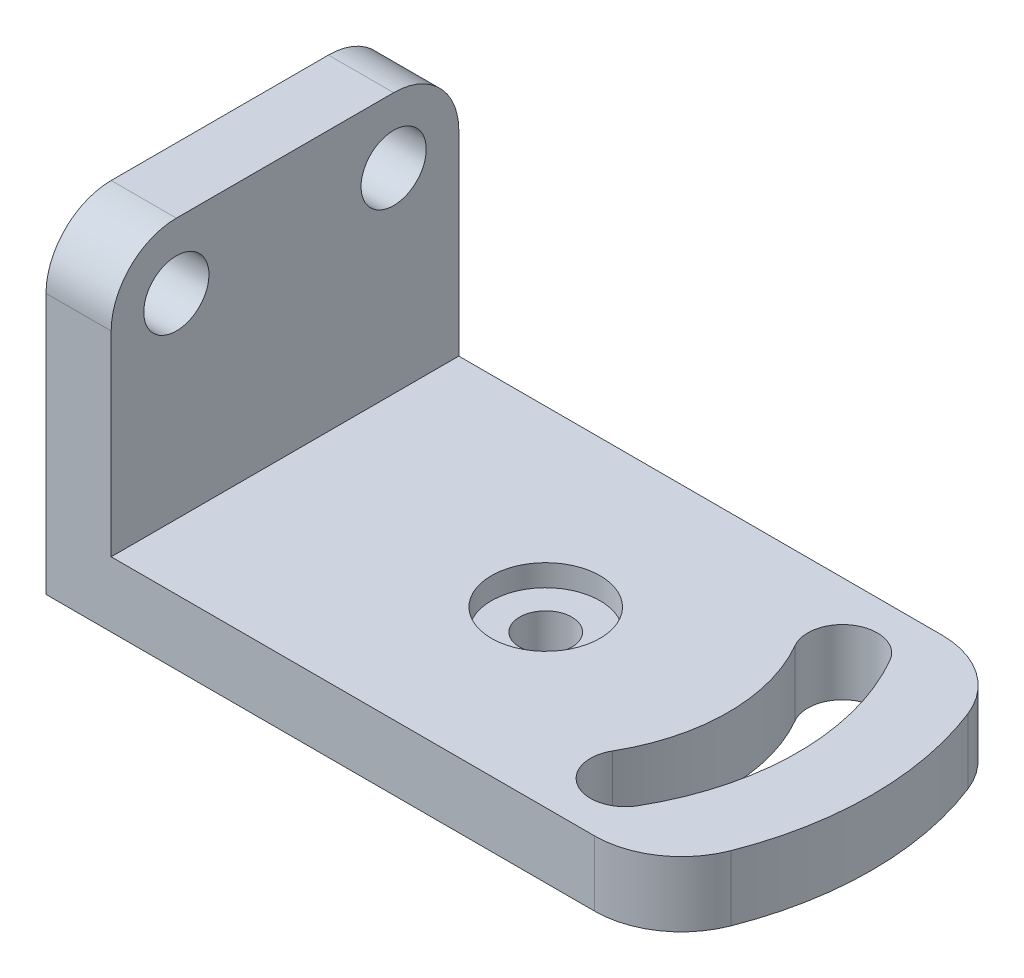
ISO-10303-21;
HEADER;
FILE_DESCRIPTION(('STEP AP214'),'2;1');
FILE_NAME('part.step','',(''),(''),'','','');
FILE_SCHEMA(('AUTOMOTIVE_DESIGN { 1 0 10303 214 1 1 1 1 }'));
ENDSEC;
DATA;
#1=APPLICATION_CONTEXT('core data for automotive mechanical design processes');
#2=APPLICATION_PROTOCOL_DEFINITION('international standard','automotive_design',2000,#1);
#3=PRODUCT_CONTEXT('',#1,'mechanical');
#4=PRODUCT('Part','Part','',(#3));
#5=PRODUCT_RELATED_PRODUCT_CATEGORY('part','',(#4));
#6=PRODUCT_DEFINITION_FORMATION('','',#4);
#7=PRODUCT_DEFINITION_CONTEXT('part definition',#1,'design');
#8=PRODUCT_DEFINITION('design','',#6,#7);
#9=PRODUCT_DEFINITION_SHAPE('','',#8);
#10=(LENGTH_UNIT() NAMED_UNIT(*) SI_UNIT(.MILLI.,.METRE.));
#11=(NAMED_UNIT(*) PLANE_ANGLE_UNIT() SI_UNIT($,.RADIAN.));
#12=(NAMED_UNIT(*) SI_UNIT($,.STERADIAN.) SOLID_ANGLE_UNIT());
#13=UNCERTAINTY_MEASURE_WITH_UNIT(LENGTH_MEASURE(1.E-05),#10,'distance_accuracy_value','');
#14=(GEOMETRIC_REPRESENTATION_CONTEXT(3) GLOBAL_UNCERTAINTY_ASSIGNED_CONTEXT((#13)) GLOBAL_UNIT_ASSIGNED_CONTEXT((#10,
#11,#12)) REPRESENTATION_CONTEXT('',''));
#15=CARTESIAN_POINT('',(0.,0.,0.));
#16=DIRECTION('',(0.,0.,1.));
#17=DIRECTION('',(1.,0.,0.));
#18=AXIS2_PLACEMENT_3D('',#15,#16,#17);
#19=CARTESIAN_POINT('',(150.,0.,40.));
#20=DIRECTION('',(0.,1.,0.));
#21=DIRECTION('',(0.,0.,1.));
#22=AXIS2_PLACEMENT_3D('',#19,#20,#21);
#23=PLANE('',#22);
#24=CARTESIAN_POINT('',(75.,0.,0.));
#25=DIRECTION('',(0.,1.,0.));
#26=DIRECTION('',(0.,0.,1.));
#27=AXIS2_PLACEMENT_3D('',#24,#25,#26);
#28=CIRCLE('',#27,6.00000000000001);
#29=CARTESIAN_POINT('',(75.,0.,6.00000000000001));
#30=VERTEX_POINT('',#29);
#31=EDGE_CURVE('E44',#30,#30,#28,.T.);
#32=ORIENTED_EDGE('',*,*,#31,.T.);
#33=EDGE_LOOP('',(#32));
#34=FACE_BOUND('',#33,.T.);
#35=CARTESIAN_POINT('',(118.301270189222,0.,25.));
#36=DIRECTION('',(0.,1.,0.));
#37=DIRECTION('',(0.,0.,1.));
#38=AXIS2_PLACEMENT_3D('',#35,#36,#37);
#39=CIRCLE('',#38,8.00000000000001);
#40=CARTESIAN_POINT('',(125.229473419497,0.,29.));
#41=VERTEX_POINT('',#40);
#42=CARTESIAN_POINT('',(111.373066958946,0.,21.));
#43=VERTEX_POINT('',#42);
#44=EDGE_CURVE('E169',#41,#43,#39,.F.);
#45=ORIENTED_EDGE('',*,*,#44,.F.);
#46=CARTESIAN_POINT('',(75.,0.,0.));
#47=DIRECTION('',(0.,1.,0.));
#48=DIRECTION('',(0.,0.,1.));
#49=AXIS2_PLACEMENT_3D('',#46,#47,#48);
#50=CIRCLE('',#49,58.);
#51=CARTESIAN_POINT('',(125.229473419497,0.,-29.));
#52=VERTEX_POINT('',#51);
#53=EDGE_CURVE('E149',#52,#41,#50,.F.);
#54=ORIENTED_EDGE('',*,*,#53,.F.);
#55=CARTESIAN_POINT('',(118.301270189222,0.,-25.0000000000001));
#56=DIRECTION('',(0.,1.,0.));
#57=DIRECTION('',(0.,0.,1.));
#58=AXIS2_PLACEMENT_3D('',#55,#56,#57);
#59=CIRCLE('',#58,8.00000000000001);
#60=CARTESIAN_POINT('',(111.373066958946,0.,-21.));
#61=VERTEX_POINT('',#60);
#62=EDGE_CURVE('E158',#61,#52,#59,.F.);
#63=ORIENTED_EDGE('',*,*,#62,.F.);
#64=CARTESIAN_POINT('',(75.,0.,0.));
#65=DIRECTION('',(0.,1.,0.));
#66=DIRECTION('',(0.,0.,1.));
#67=AXIS2_PLACEMENT_3D('',#64,#65,#66);
#68=CIRCLE('',#67,42.);
#69=EDGE_CURVE('E173',#61,#43,#68,.F.);
#70=ORIENTED_EDGE('',*,*,#69,.T.);
#71=EDGE_LOOP('',(#45,#54,#63,#70));
#72=FACE_BOUND('',#71,.T.);
#73=DIRECTION('',(1.,0.,0.));
#74=VECTOR('',#73,1.);
#75=CARTESIAN_POINT('',(150.,0.,-40.));
#76=LINE('',#75,#74);
#77=CARTESIAN_POINT('',(0.,0.,-40.));
#78=VERTEX_POINT('',#77);
#79=CARTESIAN_POINT('',(126.234753829798,0.,-40.));
#80=VERTEX_POINT('',#79);
#81=EDGE_CURVE('E192',#78,#80,#76,.T.);
#82=ORIENTED_EDGE('',*,*,#81,.T.);
#83=CARTESIAN_POINT('',(126.234753829798,0.,-20.));
#84=DIRECTION('',(0.,1.,0.));
#85=DIRECTION('',(0.,0.,1.));
#86=AXIS2_PLACEMENT_3D('',#83,#84,#85);
#87=CIRCLE('',#86,20.);
#88=CARTESIAN_POINT('',(144.86557340427,0.,-27.2727272727273));
#89=VERTEX_POINT('',#88);
#90=EDGE_CURVE('E12',#80,#89,#87,.F.);
#91=ORIENTED_EDGE('',*,*,#90,.T.);
#92=CARTESIAN_POINT('',(75.,0.,0.));
#93=DIRECTION('',(0.,1.,0.));
#94=DIRECTION('',(0.,0.,1.));
#95=AXIS2_PLACEMENT_3D('',#92,#93,#94);
#96=CIRCLE('',#95,75.);
#97=CARTESIAN_POINT('',(144.86557340427,0.,27.2727272727273));
#98=VERTEX_POINT('',#97);
#99=EDGE_CURVE('E165',#89,#98,#96,.F.);
#100=ORIENTED_EDGE('',*,*,#99,.T.);
#101=CARTESIAN_POINT('',(126.234753829798,0.,20.));
#102=DIRECTION('',(0.,1.,0.));
#103=DIRECTION('',(0.,0.,1.));
#104=AXIS2_PLACEMENT_3D('',#101,#102,#103);
#105=CIRCLE('',#104,20.);
#106=CARTESIAN_POINT('',(126.234753829798,0.,40.));
#107=VERTEX_POINT('',#106);
#108=EDGE_CURVE('E49',#98,#107,#105,.F.);
#109=ORIENTED_EDGE('',*,*,#108,.T.);
#110=DIRECTION('',(1.,0.,0.));
#111=VECTOR('',#110,1.);
#112=CARTESIAN_POINT('',(150.,0.,40.));
#113=LINE('',#112,#111);
#114=CARTESIAN_POINT('',(0.,0.,40.));
#115=VERTEX_POINT('',#114);
#116=EDGE_CURVE('E195',#115,#107,#113,.T.);
#117=ORIENTED_EDGE('',*,*,#116,.F.);
#118=DIRECTION('',(0.,0.,-1.));
#119=VECTOR('',#118,1.);
#120=CARTESIAN_POINT('',(0.,0.,40.));
#121=LINE('',#120,#119);
#122=EDGE_CURVE('E204',#115,#78,#121,.T.);
#123=ORIENTED_EDGE('',*,*,#122,.T.);
#124=EDGE_LOOP('',(#82,#91,#100,#109,#117,#123));
#125=FACE_BOUND('',#124,.T.);
#126=ADVANCED_FACE('F41',(#34,#72,#125),#23,.F.);
#127=CARTESIAN_POINT('',(15.,15.,40.));
#128=DIRECTION('',(0.,-1.,0.));
#129=DIRECTION('',(0.,0.,-1.));
#130=AXIS2_PLACEMENT_3D('',#127,#128,#129);
#131=PLANE('',#130);
#132=CARTESIAN_POINT('',(75.,15.,0.));
#133=DIRECTION('',(0.,1.,0.));
#134=DIRECTION('',(0.,0.,1.));
#135=AXIS2_PLACEMENT_3D('',#132,#133,#134);
#136=CIRCLE('',#135,12.5);
#137=CARTESIAN_POINT('',(75.,15.,12.5));
#138=VERTEX_POINT('',#137);
#139=EDGE_CURVE('E435',#138,#138,#136,.T.);
#140=ORIENTED_EDGE('',*,*,#139,.F.);
#141=EDGE_LOOP('',(#140));
#142=FACE_BOUND('',#141,.T.);
#143=CARTESIAN_POINT('',(118.301270189222,15.,-25.0000000000001));
#144=DIRECTION('',(0.,1.,0.));
#145=DIRECTION('',(0.,0.,1.));
#146=AXIS2_PLACEMENT_3D('',#143,#144,#145);
#147=CIRCLE('',#146,8.00000000000001);
#148=CARTESIAN_POINT('',(125.229473419497,15.,-29.));
#149=VERTEX_POINT('',#148);
#150=CARTESIAN_POINT('',(111.373066958946,15.,-21.));
#151=VERTEX_POINT('',#150);
#152=EDGE_CURVE('E171',#149,#151,#147,.T.);
#153=ORIENTED_EDGE('',*,*,#152,.F.);
#154=CARTESIAN_POINT('',(75.,15.,0.));
#155=DIRECTION('',(0.,1.,0.));
#156=DIRECTION('',(0.,0.,1.));
#157=AXIS2_PLACEMENT_3D('',#154,#155,#156);
#158=CIRCLE('',#157,58.);
#159=CARTESIAN_POINT('',(125.229473419497,15.,29.));
#160=VERTEX_POINT('',#159);
#161=EDGE_CURVE('E154',#160,#149,#158,.T.);
#162=ORIENTED_EDGE('',*,*,#161,.F.);
#163=CARTESIAN_POINT('',(118.301270189222,15.,25.));
#164=DIRECTION('',(0.,1.,0.));
#165=DIRECTION('',(0.,0.,1.));
#166=AXIS2_PLACEMENT_3D('',#163,#164,#165);
#167=CIRCLE('',#166,8.00000000000001);
#168=CARTESIAN_POINT('',(111.373066958946,15.,21.));
#169=VERTEX_POINT('',#168);
#170=EDGE_CURVE('E157',#169,#160,#167,.T.);
#171=ORIENTED_EDGE('',*,*,#170,.F.);
#172=CARTESIAN_POINT('',(75.,15.,0.));
#173=DIRECTION('',(0.,1.,0.));
#174=DIRECTION('',(0.,0.,1.));
#175=AXIS2_PLACEMENT_3D('',#172,#173,#174);
#176=CIRCLE('',#175,42.);
#177=EDGE_CURVE('E178',#169,#151,#176,.T.);
#178=ORIENTED_EDGE('',*,*,#177,.T.);
#179=EDGE_LOOP('',(#153,#162,#171,#178));
#180=FACE_BOUND('',#179,.T.);
#181=CARTESIAN_POINT('',(75.,15.,0.));
#182=DIRECTION('',(0.,1.,0.));
#183=DIRECTION('',(0.,0.,1.));
#184=AXIS2_PLACEMENT_3D('',#181,#182,#183);
#185=CIRCLE('',#184,75.);
#186=CARTESIAN_POINT('',(144.86557340427,15.,27.2727272727273));
#187=VERTEX_POINT('',#186);
#188=CARTESIAN_POINT('',(144.86557340427,15.,-27.2727272727273));
#189=VERTEX_POINT('',#188);
#190=EDGE_CURVE('E186',#187,#189,#185,.T.);
#191=ORIENTED_EDGE('',*,*,#190,.T.);
#192=CARTESIAN_POINT('',(126.234753829798,15.,-20.));
#193=DIRECTION('',(0.,-1.,0.));
#194=DIRECTION('',(0.,0.,-1.));
#195=AXIS2_PLACEMENT_3D('',#192,#193,#194);
#196=CIRCLE('',#195,20.);
#197=CARTESIAN_POINT('',(126.234753829798,15.,-40.));
#198=VERTEX_POINT('',#197);
#199=EDGE_CURVE('E60',#189,#198,#196,.F.);
#200=ORIENTED_EDGE('',*,*,#199,.T.);
#201=DIRECTION('',(-1.,0.,0.));
#202=VECTOR('',#201,1.);
#203=CARTESIAN_POINT('',(15.,15.,-40.));
#204=LINE('',#203,#202);
#205=CARTESIAN_POINT('',(15.,15.,-40.));
#206=VERTEX_POINT('',#205);
#207=EDGE_CURVE('E207',#198,#206,#204,.T.);
#208=ORIENTED_EDGE('',*,*,#207,.T.);
#209=DIRECTION('',(0.,0.,-1.));
#210=VECTOR('',#209,1.);
#211=CARTESIAN_POINT('',(15.,15.,40.));
#212=LINE('',#211,#210);
#213=CARTESIAN_POINT('',(15.,15.,40.));
#214=VERTEX_POINT('',#213);
#215=EDGE_CURVE('E217',#214,#206,#212,.T.);
#216=ORIENTED_EDGE('',*,*,#215,.F.);
#217=DIRECTION('',(-1.,0.,0.));
#218=VECTOR('',#217,1.);
#219=CARTESIAN_POINT('',(15.,15.,40.));
#220=LINE('',#219,#218);
#221=CARTESIAN_POINT('',(126.234753829798,15.,40.));
#222=VERTEX_POINT('',#221);
#223=EDGE_CURVE('E193',#222,#214,#220,.T.);
#224=ORIENTED_EDGE('',*,*,#223,.F.);
#225=CARTESIAN_POINT('',(126.234753829798,15.,20.));
#226=DIRECTION('',(0.,-1.,0.));
#227=DIRECTION('',(0.,0.,-1.));
#228=AXIS2_PLACEMENT_3D('',#225,#226,#227);
#229=CIRCLE('',#228,20.);
#230=EDGE_CURVE('E63',#222,#187,#229,.F.);
#231=ORIENTED_EDGE('',*,*,#230,.T.);
#232=EDGE_LOOP('',(#191,#200,#208,#216,#224,#231));
#233=FACE_BOUND('',#232,.T.);
#234=ADVANCED_FACE('F263',(#142,#180,#233),#131,.F.);
#235=CARTESIAN_POINT('',(15.,75.,40.));
#236=DIRECTION('',(-1.,0.,0.));
#237=DIRECTION('',(0.,-1.,0.));
#238=AXIS2_PLACEMENT_3D('',#235,#236,#237);
#239=PLANE('',#238);
#240=CARTESIAN_POINT('',(15.,60.,25.));
#241=DIRECTION('',(1.,0.,0.));
#242=DIRECTION('',(0.,1.,0.));
#243=AXIS2_PLACEMENT_3D('',#240,#241,#242);
#244=CIRCLE('',#243,7.5);
#245=CARTESIAN_POINT('',(15.,67.5,25.));
#246=VERTEX_POINT('',#245);
#247=EDGE_CURVE('E429',#246,#246,#244,.T.);
#248=ORIENTED_EDGE('',*,*,#247,.F.);
#249=EDGE_LOOP('',(#248));
#250=FACE_BOUND('',#249,.T.);
#251=CARTESIAN_POINT('',(15.,60.,-25.));
#252=DIRECTION('',(1.,0.,0.));
#253=DIRECTION('',(0.,1.,0.));
#254=AXIS2_PLACEMENT_3D('',#251,#252,#253);
#255=CIRCLE('',#254,7.5);
#256=CARTESIAN_POINT('',(15.,67.5,-25.));
#257=VERTEX_POINT('',#256);
#258=EDGE_CURVE('E440',#257,#257,#255,.T.);
#259=ORIENTED_EDGE('',*,*,#258,.F.);
#260=EDGE_LOOP('',(#259));
#261=FACE_BOUND('',#260,.T.);
#262=DIRECTION('',(0.,1.,0.));
#263=VECTOR('',#262,1.);
#264=CARTESIAN_POINT('',(15.,75.,-40.));
#265=LINE('',#264,#263);
#266=CARTESIAN_POINT('',(15.,60.,-40.));
#267=VERTEX_POINT('',#266);
#268=EDGE_CURVE('E206',#206,#267,#265,.T.);
#269=ORIENTED_EDGE('',*,*,#268,.T.);
#270=CARTESIAN_POINT('',(15.,60.,-25.));
#271=DIRECTION('',(-1.,0.,0.));
#272=DIRECTION('',(0.,-1.,0.));
#273=AXIS2_PLACEMENT_3D('',#270,#271,#272);
#274=CIRCLE('',#273,15.);
#275=CARTESIAN_POINT('',(15.,75.,-25.));
#276=VERTEX_POINT('',#275);
#277=EDGE_CURVE('E238',#267,#276,#274,.F.);
#278=ORIENTED_EDGE('',*,*,#277,.T.);
#279=DIRECTION('',(0.,0.,-1.));
#280=VECTOR('',#279,1.);
#281=CARTESIAN_POINT('',(15.,75.,40.));
#282=LINE('',#281,#280);
#283=CARTESIAN_POINT('',(15.,75.,25.));
#284=VERTEX_POINT('',#283);
#285=EDGE_CURVE('E216',#284,#276,#282,.T.);
#286=ORIENTED_EDGE('',*,*,#285,.F.);
#287=CARTESIAN_POINT('',(15.,60.,25.));
#288=DIRECTION('',(-1.,0.,0.));
#289=DIRECTION('',(0.,-1.,0.));
#290=AXIS2_PLACEMENT_3D('',#287,#288,#289);
#291=CIRCLE('',#290,15.);
#292=CARTESIAN_POINT('',(15.,60.,40.));
#293=VERTEX_POINT('',#292);
#294=EDGE_CURVE('E236',#284,#293,#291,.F.);
#295=ORIENTED_EDGE('',*,*,#294,.T.);
#296=DIRECTION('',(0.,1.,0.));
#297=VECTOR('',#296,1.);
#298=CARTESIAN_POINT('',(15.,75.,40.));
#299=LINE('',#298,#297);
#300=EDGE_CURVE('E200',#214,#293,#299,.T.);
#301=ORIENTED_EDGE('',*,*,#300,.F.);
#302=ORIENTED_EDGE('',*,*,#215,.T.);
#303=EDGE_LOOP('',(#269,#278,#286,#295,#301,#302));
#304=FACE_BOUND('',#303,.T.);
#305=ADVANCED_FACE('F281',(#250,#261,#304),#239,.F.);
#306=CARTESIAN_POINT('',(0.,75.,40.));
#307=DIRECTION('',(0.,-1.,0.));
#308=DIRECTION('',(1.,0.,0.));
#309=AXIS2_PLACEMENT_3D('',#306,#307,#308);
#310=PLANE('',#309);
#311=ORIENTED_EDGE('',*,*,#285,.T.);
#312=DIRECTION('',(-1.,0.,0.));
#313=VECTOR('',#312,1.);
#314=CARTESIAN_POINT('',(0.,75.,-25.));
#315=LINE('',#314,#313);
#316=CARTESIAN_POINT('',(0.,75.,-25.));
#317=VERTEX_POINT('',#316);
#318=EDGE_CURVE('E223',#276,#317,#315,.T.);
#319=ORIENTED_EDGE('',*,*,#318,.T.);
#320=DIRECTION('',(0.,0.,-1.));
#321=VECTOR('',#320,1.);
#322=CARTESIAN_POINT('',(0.,75.,40.));
#323=LINE('',#322,#321);
#324=CARTESIAN_POINT('',(0.,75.,25.));
#325=VERTEX_POINT('',#324);
#326=EDGE_CURVE('E211',#325,#317,#323,.T.);
#327=ORIENTED_EDGE('',*,*,#326,.F.);
#328=DIRECTION('',(-1.,0.,0.));
#329=VECTOR('',#328,1.);
#330=CARTESIAN_POINT('',(0.,75.,25.));
#331=LINE('',#330,#329);
#332=EDGE_CURVE('E224',#325,#284,#331,.F.);
#333=ORIENTED_EDGE('',*,*,#332,.T.);
#334=EDGE_LOOP('',(#311,#319,#327,#333));
#335=FACE_BOUND('',#334,.T.);
#336=ADVANCED_FACE('F282',(#335),#310,.F.);
#337=CARTESIAN_POINT('',(0.,0.,40.));
#338=DIRECTION('',(1.,0.,0.));
#339=DIRECTION('',(0.,0.,-1.));
#340=AXIS2_PLACEMENT_3D('',#337,#338,#339);
#341=PLANE('',#340);
#342=CARTESIAN_POINT('',(0.,60.,25.));
#343=DIRECTION('',(1.,0.,0.));
#344=DIRECTION('',(0.,0.,-1.));
#345=AXIS2_PLACEMENT_3D('',#342,#343,#344);
#346=CIRCLE('',#345,7.5);
#347=CARTESIAN_POINT('',(0.,60.,17.5));
#348=VERTEX_POINT('',#347);
#349=EDGE_CURVE('E431',#348,#348,#346,.F.);
#350=ORIENTED_EDGE('',*,*,#349,.F.);
#351=EDGE_LOOP('',(#350));
#352=FACE_BOUND('',#351,.T.);
#353=CARTESIAN_POINT('',(0.,60.,-25.));
#354=DIRECTION('',(1.,0.,0.));
#355=DIRECTION('',(0.,0.,-1.));
#356=AXIS2_PLACEMENT_3D('',#353,#354,#355);
#357=CIRCLE('',#356,7.5);
#358=CARTESIAN_POINT('',(0.,60.,-32.5));
#359=VERTEX_POINT('',#358);
#360=EDGE_CURVE('E439',#359,#359,#357,.F.);
#361=ORIENTED_EDGE('',*,*,#360,.F.);
#362=EDGE_LOOP('',(#361));
#363=FACE_BOUND('',#362,.T.);
#364=ORIENTED_EDGE('',*,*,#326,.T.);
#365=CARTESIAN_POINT('',(0.,60.,-25.));
#366=DIRECTION('',(1.,0.,0.));
#367=DIRECTION('',(0.,0.,-1.));
#368=AXIS2_PLACEMENT_3D('',#365,#366,#367);
#369=CIRCLE('',#368,15.);
#370=CARTESIAN_POINT('',(0.,60.,-40.));
#371=VERTEX_POINT('',#370);
#372=EDGE_CURVE('E229',#317,#371,#369,.F.);
#373=ORIENTED_EDGE('',*,*,#372,.T.);
#374=DIRECTION('',(0.,-1.,0.));
#375=VECTOR('',#374,1.);
#376=CARTESIAN_POINT('',(0.,0.,-40.));
#377=LINE('',#376,#375);
#378=EDGE_CURVE('E199',#371,#78,#377,.T.);
#379=ORIENTED_EDGE('',*,*,#378,.T.);
#380=ORIENTED_EDGE('',*,*,#122,.F.);
#381=DIRECTION('',(0.,-1.,0.));
#382=VECTOR('',#381,1.);
#383=CARTESIAN_POINT('',(0.,0.,40.));
#384=LINE('',#383,#382);
#385=CARTESIAN_POINT('',(0.,60.,40.));
#386=VERTEX_POINT('',#385);
#387=EDGE_CURVE('E202',#386,#115,#384,.T.);
#388=ORIENTED_EDGE('',*,*,#387,.F.);
#389=CARTESIAN_POINT('',(0.,60.,25.));
#390=DIRECTION('',(1.,0.,0.));
#391=DIRECTION('',(0.,0.,-1.));
#392=AXIS2_PLACEMENT_3D('',#389,#390,#391);
#393=CIRCLE('',#392,15.);
#394=EDGE_CURVE('E226',#386,#325,#393,.F.);
#395=ORIENTED_EDGE('',*,*,#394,.T.);
#396=EDGE_LOOP('',(#364,#373,#379,#380,#388,#395));
#397=FACE_BOUND('',#396,.T.);
#398=ADVANCED_FACE('F292',(#352,#363,#397),#341,.F.);
#399=CARTESIAN_POINT('',(0.,0.,40.));
#400=DIRECTION('',(0.,0.,-1.));
#401=DIRECTION('',(-1.,0.,0.));
#402=AXIS2_PLACEMENT_3D('',#399,#400,#401);
#403=PLANE('',#402);
#404=ORIENTED_EDGE('',*,*,#300,.T.);
#405=DIRECTION('',(-1.,0.,0.));
#406=VECTOR('',#405,1.);
#407=CARTESIAN_POINT('',(0.,60.,40.));
#408=LINE('',#407,#406);
#409=EDGE_CURVE('E243',#293,#386,#408,.T.);
#410=ORIENTED_EDGE('',*,*,#409,.T.);
#411=ORIENTED_EDGE('',*,*,#387,.T.);
#412=ORIENTED_EDGE('',*,*,#116,.T.);
#413=DIRECTION('',(0.,-1.,0.));
#414=VECTOR('',#413,1.);
#415=CARTESIAN_POINT('',(126.234753829798,15.,40.));
#416=LINE('',#415,#414);
#417=EDGE_CURVE('E239',#107,#222,#416,.F.);
#418=ORIENTED_EDGE('',*,*,#417,.T.);
#419=ORIENTED_EDGE('',*,*,#223,.T.);
#420=EDGE_LOOP('',(#404,#410,#411,#412,#418,#419));
#421=FACE_BOUND('',#420,.T.);
#422=ADVANCED_FACE('F256',(#421),#403,.F.);
#423=CARTESIAN_POINT('',(0.,0.,-40.));
#424=DIRECTION('',(0.,0.,-1.));
#425=DIRECTION('',(-1.,0.,0.));
#426=AXIS2_PLACEMENT_3D('',#423,#424,#425);
#427=PLANE('',#426);
#428=ORIENTED_EDGE('',*,*,#378,.F.);
#429=DIRECTION('',(-1.,0.,0.));
#430=VECTOR('',#429,1.);
#431=CARTESIAN_POINT('',(15.,60.,-40.));
#432=LINE('',#431,#430);
#433=EDGE_CURVE('E234',#371,#267,#432,.F.);
#434=ORIENTED_EDGE('',*,*,#433,.T.);
#435=ORIENTED_EDGE('',*,*,#268,.F.);
#436=ORIENTED_EDGE('',*,*,#207,.F.);
#437=DIRECTION('',(0.,1.,0.));
#438=VECTOR('',#437,1.);
#439=CARTESIAN_POINT('',(126.234753829798,0.,-40.));
#440=LINE('',#439,#438);
#441=EDGE_CURVE('E235',#198,#80,#440,.F.);
#442=ORIENTED_EDGE('',*,*,#441,.T.);
#443=ORIENTED_EDGE('',*,*,#81,.F.);
#444=EDGE_LOOP('',(#428,#434,#435,#436,#442,#443));
#445=FACE_BOUND('',#444,.T.);
#446=ADVANCED_FACE('F268',(#445),#427,.T.);
#447=CARTESIAN_POINT('',(75.,-0.000999999999999265,0.));
#448=DIRECTION('',(0.,1.,0.));
#449=DIRECTION('',(0.,0.,1.));
#450=AXIS2_PLACEMENT_3D('',#447,#448,#449);
#451=CYLINDRICAL_SURFACE('',#450,75.);
#452=ORIENTED_EDGE('',*,*,#99,.F.);
#453=DIRECTION('',(0.,1.,0.));
#454=VECTOR('',#453,1.);
#455=CARTESIAN_POINT('',(144.86557340427,-0.000999999999999265,-27.2727272727273));
#456=LINE('',#455,#454);
#457=EDGE_CURVE('E247',#89,#189,#456,.T.);
#458=ORIENTED_EDGE('',*,*,#457,.T.);
#459=ORIENTED_EDGE('',*,*,#190,.F.);
#460=DIRECTION('',(0.,1.,0.));
#461=VECTOR('',#460,1.);
#462=CARTESIAN_POINT('',(144.86557340427,-0.000999999999999265,27.2727272727273));
#463=LINE('',#462,#461);
#464=EDGE_CURVE('E246',#187,#98,#463,.F.);
#465=ORIENTED_EDGE('',*,*,#464,.T.);
#466=EDGE_LOOP('',(#452,#458,#459,#465));
#467=FACE_BOUND('',#466,.T.);
#468=ADVANCED_FACE('F265',(#467),#451,.T.);
#469=CARTESIAN_POINT('',(75.,-0.000999999999999265,0.));
#470=DIRECTION('',(0.,1.,0.));
#471=DIRECTION('',(0.,0.,1.));
#472=AXIS2_PLACEMENT_3D('',#469,#470,#471);
#473=CYLINDRICAL_SURFACE('',#472,58.);
#474=ORIENTED_EDGE('',*,*,#53,.T.);
#475=DIRECTION('',(0.,1.,0.));
#476=VECTOR('',#475,1.);
#477=CARTESIAN_POINT('',(125.229473419497,-0.000999999999999265,29.));
#478=LINE('',#477,#476);
#479=EDGE_CURVE('E164',#41,#160,#478,.T.);
#480=ORIENTED_EDGE('',*,*,#479,.T.);
#481=ORIENTED_EDGE('',*,*,#161,.T.);
#482=DIRECTION('',(0.,1.,0.));
#483=VECTOR('',#482,1.);
#484=CARTESIAN_POINT('',(125.229473419497,-0.000999999999999265,-29.));
#485=LINE('',#484,#483);
#486=EDGE_CURVE('E144',#52,#149,#485,.T.);
#487=ORIENTED_EDGE('',*,*,#486,.F.);
#488=EDGE_LOOP('',(#474,#480,#481,#487));
#489=FACE_BOUND('',#488,.T.);
#490=ADVANCED_FACE('F147',(#489),#473,.F.);
#491=CARTESIAN_POINT('',(118.301270189222,-0.000999999999999265,25.));
#492=DIRECTION('',(0.,1.,0.));
#493=DIRECTION('',(0.,0.,1.));
#494=AXIS2_PLACEMENT_3D('',#491,#492,#493);
#495=CYLINDRICAL_SURFACE('',#494,8.00000000000001);
#496=ORIENTED_EDGE('',*,*,#44,.T.);
#497=DIRECTION('',(0.,1.,0.));
#498=VECTOR('',#497,1.);
#499=CARTESIAN_POINT('',(111.373066958946,-0.000999999999999265,21.));
#500=LINE('',#499,#498);
#501=EDGE_CURVE('E183',#43,#169,#500,.T.);
#502=ORIENTED_EDGE('',*,*,#501,.T.);
#503=ORIENTED_EDGE('',*,*,#170,.T.);
#504=ORIENTED_EDGE('',*,*,#479,.F.);
#505=EDGE_LOOP('',(#496,#502,#503,#504));
#506=FACE_BOUND('',#505,.T.);
#507=ADVANCED_FACE('F345',(#506),#495,.F.);
#508=CARTESIAN_POINT('',(75.,-0.000999999999999265,0.));
#509=DIRECTION('',(0.,1.,0.));
#510=DIRECTION('',(0.,0.,1.));
#511=AXIS2_PLACEMENT_3D('',#508,#509,#510);
#512=CYLINDRICAL_SURFACE('',#511,42.);
#513=DIRECTION('',(0.,1.,0.));
#514=VECTOR('',#513,1.);
#515=CARTESIAN_POINT('',(111.373066958946,-0.000999999999999265,-21.));
#516=LINE('',#515,#514);
#517=EDGE_CURVE('E152',#61,#151,#516,.T.);
#518=ORIENTED_EDGE('',*,*,#517,.T.);
#519=ORIENTED_EDGE('',*,*,#177,.F.);
#520=ORIENTED_EDGE('',*,*,#501,.F.);
#521=ORIENTED_EDGE('',*,*,#69,.F.);
#522=EDGE_LOOP('',(#518,#519,#520,#521));
#523=FACE_BOUND('',#522,.T.);
#524=ADVANCED_FACE('F343',(#523),#512,.T.);
#525=CARTESIAN_POINT('',(118.301270189222,-0.000999999999999265,-25.0000000000001));
#526=DIRECTION('',(0.,1.,0.));
#527=DIRECTION('',(0.,0.,1.));
#528=AXIS2_PLACEMENT_3D('',#525,#526,#527);
#529=CYLINDRICAL_SURFACE('',#528,8.00000000000001);
#530=ORIENTED_EDGE('',*,*,#62,.T.);
#531=ORIENTED_EDGE('',*,*,#486,.T.);
#532=ORIENTED_EDGE('',*,*,#152,.T.);
#533=ORIENTED_EDGE('',*,*,#517,.F.);
#534=EDGE_LOOP('',(#530,#531,#532,#533));
#535=FACE_BOUND('',#534,.T.);
#536=ADVANCED_FACE('F163',(#535),#529,.F.);
#537=CARTESIAN_POINT('',(0.,60.,-25.));
#538=DIRECTION('',(1.,0.,0.));
#539=DIRECTION('',(0.,1.,0.));
#540=AXIS2_PLACEMENT_3D('',#537,#538,#539);
#541=CYLINDRICAL_SURFACE('',#540,15.);
#542=ORIENTED_EDGE('',*,*,#277,.F.);
#543=ORIENTED_EDGE('',*,*,#433,.F.);
#544=ORIENTED_EDGE('',*,*,#372,.F.);
#545=ORIENTED_EDGE('',*,*,#318,.F.);
#546=EDGE_LOOP('',(#542,#543,#544,#545));
#547=FACE_BOUND('',#546,.T.);
#548=ADVANCED_FACE('F279',(#547),#541,.T.);
#549=CARTESIAN_POINT('',(0.,60.,25.));
#550=DIRECTION('',(-1.,0.,0.));
#551=DIRECTION('',(0.,-1.,0.));
#552=AXIS2_PLACEMENT_3D('',#549,#550,#551);
#553=CYLINDRICAL_SURFACE('',#552,15.);
#554=ORIENTED_EDGE('',*,*,#294,.F.);
#555=ORIENTED_EDGE('',*,*,#332,.F.);
#556=ORIENTED_EDGE('',*,*,#394,.F.);
#557=ORIENTED_EDGE('',*,*,#409,.F.);
#558=EDGE_LOOP('',(#554,#555,#556,#557));
#559=FACE_BOUND('',#558,.T.);
#560=ADVANCED_FACE('F286',(#559),#553,.T.);
#561=CARTESIAN_POINT('',(126.234753829798,-0.000999999999999265,-20.));
#562=DIRECTION('',(0.,1.,0.));
#563=DIRECTION('',(0.,0.,1.));
#564=AXIS2_PLACEMENT_3D('',#561,#562,#563);
#565=CYLINDRICAL_SURFACE('',#564,20.);
#566=ORIENTED_EDGE('',*,*,#90,.F.);
#567=ORIENTED_EDGE('',*,*,#441,.F.);
#568=ORIENTED_EDGE('',*,*,#199,.F.);
#569=ORIENTED_EDGE('',*,*,#457,.F.);
#570=EDGE_LOOP('',(#566,#567,#568,#569));
#571=FACE_BOUND('',#570,.T.);
#572=ADVANCED_FACE('F271',(#571),#565,.T.);
#573=CARTESIAN_POINT('',(126.234753829798,-0.000999999999999265,20.));
#574=DIRECTION('',(0.,1.,0.));
#575=DIRECTION('',(0.,0.,1.));
#576=AXIS2_PLACEMENT_3D('',#573,#574,#575);
#577=CYLINDRICAL_SURFACE('',#576,20.);
#578=ORIENTED_EDGE('',*,*,#108,.F.);
#579=ORIENTED_EDGE('',*,*,#464,.F.);
#580=ORIENTED_EDGE('',*,*,#230,.F.);
#581=ORIENTED_EDGE('',*,*,#417,.F.);
#582=EDGE_LOOP('',(#578,#579,#580,#581));
#583=FACE_BOUND('',#582,.T.);
#584=ADVANCED_FACE('F43',(#583),#577,.T.);
#585=CARTESIAN_POINT('',(75.,15.,0.));
#586=DIRECTION('',(0.,1.,0.));
#587=DIRECTION('',(0.,0.,1.));
#588=AXIS2_PLACEMENT_3D('',#585,#586,#587);
#589=CYLINDRICAL_SURFACE('',#588,6.00000000000001);
#590=CARTESIAN_POINT('',(75.,10.,0.));
#591=DIRECTION('',(0.,1.,0.));
#592=DIRECTION('',(0.,0.,1.));
#593=AXIS2_PLACEMENT_3D('',#590,#591,#592);
#594=CIRCLE('',#593,6.00000000000002);
#595=CARTESIAN_POINT('',(75.,10.,6.00000000000002));
#596=VERTEX_POINT('',#595);
#597=EDGE_CURVE('E450',#596,#596,#594,.T.);
#598=ORIENTED_EDGE('',*,*,#597,.T.);
#599=EDGE_LOOP('',(#598));
#600=FACE_BOUND('',#599,.T.);
#601=ORIENTED_EDGE('',*,*,#31,.F.);
#602=EDGE_LOOP('',(#601));
#603=FACE_BOUND('',#602,.T.);
#604=ADVANCED_FACE('F323',(#600,#603),#589,.F.);
#605=CARTESIAN_POINT('',(81.,10.,0.));
#606=DIRECTION('',(0.,-1.,0.));
#607=DIRECTION('',(0.,0.,-1.));
#608=AXIS2_PLACEMENT_3D('',#605,#606,#607);
#609=PLANE('',#608);
#610=ORIENTED_EDGE('',*,*,#597,.F.);
#611=EDGE_LOOP('',(#610));
#612=FACE_BOUND('',#611,.T.);
#613=CARTESIAN_POINT('',(75.,10.,0.));
#614=DIRECTION('',(0.,1.,0.));
#615=DIRECTION('',(0.,0.,1.));
#616=AXIS2_PLACEMENT_3D('',#613,#614,#615);
#617=CIRCLE('',#616,12.5);
#618=CARTESIAN_POINT('',(75.,10.,12.5));
#619=VERTEX_POINT('',#618);
#620=EDGE_CURVE('E434',#619,#619,#617,.T.);
#621=ORIENTED_EDGE('',*,*,#620,.T.);
#622=EDGE_LOOP('',(#621));
#623=FACE_BOUND('',#622,.T.);
#624=ADVANCED_FACE('F328',(#612,#623),#609,.F.);
#625=CARTESIAN_POINT('',(75.,15.,0.));
#626=DIRECTION('',(0.,1.,0.));
#627=DIRECTION('',(0.,0.,1.));
#628=AXIS2_PLACEMENT_3D('',#625,#626,#627);
#629=CYLINDRICAL_SURFACE('',#628,12.5);
#630=ORIENTED_EDGE('',*,*,#620,.F.);
#631=EDGE_LOOP('',(#630));
#632=FACE_BOUND('',#631,.T.);
#633=ORIENTED_EDGE('',*,*,#139,.T.);
#634=EDGE_LOOP('',(#633));
#635=FACE_BOUND('',#634,.T.);
#636=ADVANCED_FACE('F333',(#632,#635),#629,.F.);
#637=CARTESIAN_POINT('',(-0.0010000000000062,60.,-25.));
#638=DIRECTION('',(1.,0.,0.));
#639=DIRECTION('',(0.,1.,0.));
#640=AXIS2_PLACEMENT_3D('',#637,#638,#639);
#641=CYLINDRICAL_SURFACE('',#640,7.5);
#642=ORIENTED_EDGE('',*,*,#258,.T.);
#643=EDGE_LOOP('',(#642));
#644=FACE_BOUND('',#643,.T.);
#645=ORIENTED_EDGE('',*,*,#360,.T.);
#646=EDGE_LOOP('',(#645));
#647=FACE_BOUND('',#646,.T.);
#648=ADVANCED_FACE('F403',(#644,#647),#641,.F.);
#649=CARTESIAN_POINT('',(-0.0010000000000062,60.,25.));
#650=DIRECTION('',(1.,0.,0.));
#651=DIRECTION('',(0.,1.,0.));
#652=AXIS2_PLACEMENT_3D('',#649,#650,#651);
#653=CYLINDRICAL_SURFACE('',#652,7.5);
#654=ORIENTED_EDGE('',*,*,#247,.T.);
#655=EDGE_LOOP('',(#654));
#656=FACE_BOUND('',#655,.T.);
#657=ORIENTED_EDGE('',*,*,#349,.T.);
#658=EDGE_LOOP('',(#657));
#659=FACE_BOUND('',#658,.T.);
#660=ADVANCED_FACE('F415',(#656,#659),#653,.F.);
#661=CLOSED_SHELL('',(#126,#234,#305,#336,#398,#422,#446,#468,#490,#507,#524,#536,#548,#560,
#572,#584,#604,#624,#636,#648,#660));
#662=MANIFOLD_SOLID_BREP('B2',#661);
#663=ADVANCED_BREP_SHAPE_REPRESENTATION('',(#18,#662),#14);
#664=SHAPE_DEFINITION_REPRESENTATION(#9,#663);
ENDSEC;
END-ISO-10303-21;
